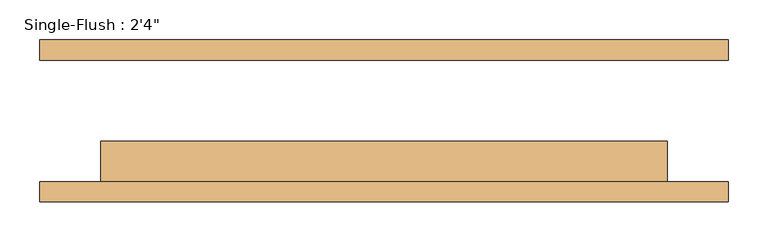
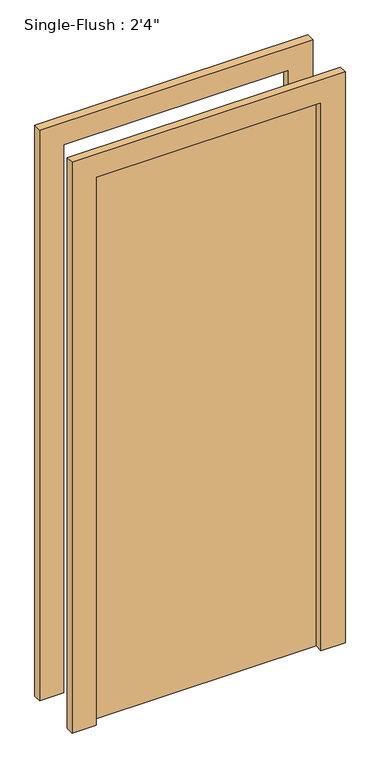
"""IFC4 building model written with IfcOpenShell, lengths in millimetres: door geometry."""

from ifc_helpers import new_model, si_unit, frame, origin, origin_with_axes, place, context, project, spatial, polyline, outline, extrude, source, transform, mapped, element, save


def door_77f51d0b(model_context):
    return source(origin(), model_context, "Body", "SweptSolid", [
        extrude(outline(polyline([(1905.0, -431.8), (0.0, -431.8), (0.0, -355.6), (1828.8, -355.6), (1828.8, 355.6), (0.0, 355.6), (0.0, 431.8), (1905.0, 431.8), (1905.0, -431.8)])), frame((0.0, -101.6, 0.0), z_axis=(0.0, 1.0, 0.0), x_axis=(0.0, 0.0, 1.0)), (0.0, 0.0, 1.0), 25.4),
        extrude(outline(polyline([(1905.0, 431.8), (1905.0, -431.8), (0.0, -431.8), (0.0, -355.6), (1828.8, -355.6), (1828.8, 355.6), (0.0, 355.6), (0.0, 431.8), (1905.0, 431.8)])), frame((0.0, 76.2, 0.0), z_axis=(0.0, 1.0, 0.0), x_axis=(0.0, 0.0, 1.0)), (0.0, 0.0, 1.0), 25.4),
        extrude(outline(polyline([(355.6, -25.4), (355.6, -76.2), (-355.6, -76.2), (-355.6, -25.4), (355.6, -25.4)])), origin_with_axes(), (0.0, 0.0, 1.0), 1828.8),
    ])


if __name__ == "__main__":
    model = new_model("IFC4")
    model_context = context("Model", 3, world=origin())
    ifc_project = project(units=[si_unit("LENGTHUNIT", "METRE", prefix="MILLI")], contexts=[model_context])
    site = spatial("IfcSite", under=ifc_project)
    building = spatial("IfcBuilding", under=site)
    placement = place(None, origin())
    door_shape = door_77f51d0b(model_context)
    element("IfcDoor", 1, ObjectType="Single-Flush : 2'4\"", at=placement, inside=building, context=model_context, shape_type="MappedRepresentation", body=[
        mapped(door_shape, transform((0.0, 0.0, 0.0), x_axis=(1.0, 0.0, 0.0), y_axis=(0.0, 1.0, 0.0), z_axis=(0.0, 0.0, 1.0))),
    ])
    save(model, "model.ifc")

# Revit data of these elements
# Type "Single-Flush : 2'4\""
#   Type Mark = "10"
#   Construction Type Id = "MDOOR"
#   Assembly Code = "C1020"
#   Analytic Construction = "Metal"
#   Thickness = 0' - 2"
#   Heat Transfer Coefficient (U) = 0.651978 BTU/(h·ft²·°F)
#   Height = 6' - 0"
#   Trim Projection Ext = 0' - 1"
#   Trim Projection Int = 0' - 1"
#   Trim Width = 0' - 3"
#   Width = 2' - 4"
#   Define Thermal Properties by = 1
#   Door Material = Door - Panel
#   Frame Material = Door - Frame
#   Visual Light Transmittance = 0
#   Solar Heat Gain Coefficient = 0
#   Function = (empty or 0)
#   Wall Closure = (empty or 0)
# Element 1 (IfcDoor, "Single-Flush : 2'4\"")
#   Materials on its faces: "Door - Frame", "Door - Panel"
# Materials
#   "Door - Panel": class "Wood", colour RGB 210 159 95, transparency 0, Cost = 0
#   "Door - Frame": colour RGB 118 70 51, transparency 0, Cost = 0
